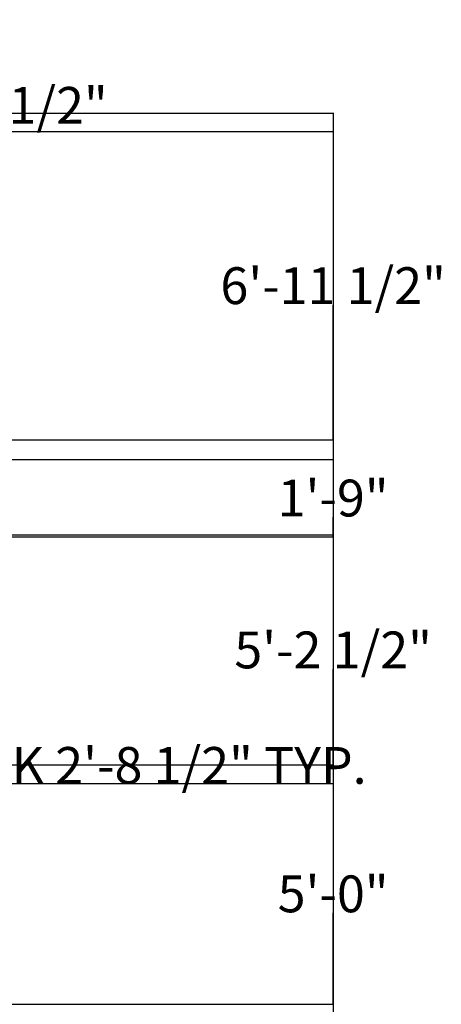
# Model space of a CAD drawing. Units: inches. Extents: x 541 to 1172, y -20 to 887.
# Tile 8 of 8: x 1058 to 1172, y 588 to 855. Entities that reach past the tile are written whole.
import ezdxf

# ---------------------------------------------------------------- set-up
doc = ezdxf.new("R2010")
doc.units = ezdxf.units.IN
doc.header["$MEASUREMENT"] = 0
doc.layers.add('A-ANNO-DIMS', color=2, linetype='Continuous', lineweight=18)
doc.styles.get("Standard").update_dxf_attribs({"font": 'arial.ttf'})
doc.dimstyles.get("Standard").update_dxf_attribs({"dimtxt": 10, "dimasz": 0.18, "dimexe": 0.18, "dimexo": 0.0625, "dimgap": 0.09, "dimtad": 0, "dimtih": 1, "dimtoh": 1, "dimdec": 1, "dimzin": 0, "dimdsep": 46, "dimlunit": 4, "dimtxsty": 'Standard', "dimcen": 0.09, "dimadec": 0, "dimazin": 0, "dimtfac": 1, "dimtdec": 1, "dimtofl": 0, "dimtmove": 0, "dimatfit": 3, "dimfxl": 1, "dimtolj": 1, "dimtzin": 0, "dimarcsym": 0})

# ---------------------------------------------------------------- blocks, each defined once
blk = doc.blocks.new('*D51')
at = {"layer": 'A-ANNO-DIMS', "color": 0, "lineweight": -2, "transparency": 16777216}
for p, q in [((999.81, 647.72), (999.81, 652.71)), ((999.99, 652.53), (1032.1, 652.53)), ((1032.28, 647.72), (1032.28, 652.71)), ((1032.28, 652.53), (1032.46, 652.53))]:
    blk.add_line(p, q, dxfattribs=at)
for points in [[(999.99, 652.56), (999.99, 652.5), (999.81, 652.53)], [(1032.1, 652.56), (1032.1, 652.5), (1032.28, 652.53)]]:
    blk.add_solid(points, dxfattribs=at)
at = {"layer": 'Defpoints', "color": 0, "lineweight": -2, "transparency": 16777216}
for p in [(1032.28, 652.53), (999.81, 647.65), (1032.28, 647.65)]:
    blk.add_point(p, dxfattribs=at)
at = {"layer": 'A-ANNO-DIMS', "color": 0, "transparency": 16777216, "insert": (1092.9, 652.53), "char_height": 10, "attachment_point": 5}
blk.add_mtext('\\A1;SINK 2\'-8 1/2" TYP.', dxfattribs=at)
blk = doc.blocks.new('*D53')
at = {"layer": 'A-ANNO-DIMS', "color": 0, "lineweight": -2, "transparency": 16777216}
for p, q in [((940.56, 824.91), (940.56, 831.98)), ((940.74, 831.8), (986.74, 831.8)), ((986.92, 824.91), (986.92, 831.98)), ((986.92, 831.8), (987.1, 831.8))]:
    blk.add_line(p, q, dxfattribs=at)
for points in [[(940.74, 831.83), (940.74, 831.77), (940.56, 831.8)], [(986.74, 831.83), (986.74, 831.77), (986.92, 831.8)]]:
    blk.add_solid(points, dxfattribs=at)
at = {"layer": 'Defpoints', "color": 0, "lineweight": -2, "transparency": 16777216}
for p in [(986.92, 831.8), (940.56, 824.85), (986.92, 824.85)]:
    blk.add_point(p, dxfattribs=at)
at = {"layer": 'A-ANNO-DIMS', "color": 0, "transparency": 16777216, "insert": (1034.24, 831.8), "char_height": 10, "attachment_point": 5}
blk.add_mtext('\\A1;SINK 3\'-10 1/2"', dxfattribs=at)
blk = doc.blocks.new('*D70')
at = {"layer": 'A-ANNO-DIMS', "color": 0, "lineweight": -2, "transparency": 16777216}
for p, q in [((1036.7, 829.68), (1143.21, 829.68)), ((1143.03, 829.5), (1143.03, 444.36)), ((1143.03, 48.83), (1143.03, 433.97)), ((1037.35, 48.65), (1143.21, 48.65))]:
    blk.add_line(p, q, dxfattribs=at)
for points in [[(1143, 829.5), (1143.06, 829.5), (1143.03, 829.68)], [(1143, 48.83), (1143.06, 48.83), (1143.03, 48.65)]]:
    blk.add_solid(points, dxfattribs=at)
at = {"layer": 'Defpoints', "color": 0, "lineweight": -2, "transparency": 16777216}
for p in [(1036.64, 829.68), (1037.28, 48.65), (1143.03, 48.65)]:
    blk.add_point(p, dxfattribs=at)
at = {"layer": 'A-ANNO-DIMS', "color": 0, "transparency": 16777216, "insert": (1143.03, 439.17), "char_height": 10, "attachment_point": 5}
blk.add_mtext('\\A1;65\'-1"', dxfattribs=at)
blk = doc.blocks.new('*D79')
at = {"layer": 'A-ANNO-DIMS', "color": 0, "lineweight": -2, "transparency": 16777216}
for p, q in [((1031.73, 824.68), (1143.21, 824.68)), ((1143.03, 824.5), (1143.03, 788.09)), ((1143.03, 741.17), (1143.03, 777.57)), ((1032.19, 740.99), (1143.21, 740.99))]:
    blk.add_line(p, q, dxfattribs=at)
for points in [[(1143, 824.5), (1143.06, 824.5), (1143.03, 824.68)], [(1143, 741.17), (1143.06, 741.17), (1143.03, 740.99)]]:
    blk.add_solid(points, dxfattribs=at)
at = {"layer": 'Defpoints', "color": 0, "lineweight": -2, "transparency": 16777216}
for p in [(1031.66, 824.68), (1032.13, 740.99), (1143.03, 740.99)]:
    blk.add_point(p, dxfattribs=at)
at = {"layer": 'A-ANNO-DIMS', "color": 0, "transparency": 16777216, "insert": (1143.03, 782.83), "char_height": 10, "attachment_point": 5}
blk.add_mtext('\\A1;6\'-11 1/2"', dxfattribs=at)
blk = doc.blocks.new('*D80')
at = {"layer": 'A-ANNO-DIMS', "color": 0, "lineweight": -2, "transparency": 16777216}
for p, q in [((1032.33, 715.15), (1143.21, 715.15)), ((1143.03, 714.97), (1143.03, 689.16)), ((1143.03, 652.83), (1143.03, 678.64)), ((1032.35, 652.65), (1143.21, 652.65))]:
    blk.add_line(p, q, dxfattribs=at)
for points in [[(1143, 714.97), (1143.06, 714.97), (1143.03, 715.15)], [(1143, 652.83), (1143.06, 652.83), (1143.03, 652.65)]]:
    blk.add_solid(points, dxfattribs=at)
at = {"layer": 'Defpoints', "color": 0, "lineweight": -2, "transparency": 16777216}
for p in [(1032.27, 715.15), (1032.28, 652.65), (1143.03, 652.65)]:
    blk.add_point(p, dxfattribs=at)
at = {"layer": 'A-ANNO-DIMS', "color": 0, "transparency": 16777216, "insert": (1143.03, 683.9), "char_height": 10, "attachment_point": 5}
blk.add_mtext('\\A1;5\'-2 1/2"', dxfattribs=at)
blk = doc.blocks.new('*D81')
at = {"layer": 'A-ANNO-DIMS', "color": 0, "lineweight": -2, "transparency": 16777216}
for p, q in [((1032.35, 647.65), (1143.21, 647.65)), ((1143.03, 647.47), (1143.03, 622.85)), ((1143.03, 587.83), (1143.03, 612.46)), ((1032.35, 587.65), (1143.21, 587.65))]:
    blk.add_line(p, q, dxfattribs=at)
for points in [[(1143, 647.47), (1143.06, 647.47), (1143.03, 647.65)], [(1143, 587.83), (1143.06, 587.83), (1143.03, 587.65)]]:
    blk.add_solid(points, dxfattribs=at)
at = {"layer": 'Defpoints', "color": 0, "lineweight": -2, "transparency": 16777216}
for p in [(1032.28, 647.65), (1032.28, 587.65), (1143.03, 587.65)]:
    blk.add_point(p, dxfattribs=at)
at = {"layer": 'A-ANNO-DIMS', "color": 0, "transparency": 16777216, "insert": (1143.03, 617.65), "char_height": 10, "attachment_point": 5}
blk.add_mtext('\\A1;5\'-0"', dxfattribs=at)
blk = doc.blocks.new('*D101')
at = {"layer": 'A-ANNO-DIMS', "color": 0, "lineweight": -2, "transparency": 16777216}
for p, q in [((805.35, 735.65), (1143.21, 735.65)), ((1143.03, 735.47), (1143.03, 730.35)), ((1143.03, 714.83), (1143.03, 719.96)), ((805.35, 714.65), (1143.21, 714.65))]:
    blk.add_line(p, q, dxfattribs=at)
for points in [[(1143, 735.47), (1143.06, 735.47), (1143.03, 735.65)], [(1143, 714.83), (1143.06, 714.83), (1143.03, 714.65)]]:
    blk.add_solid(points, dxfattribs=at)
at = {"layer": 'Defpoints', "color": 0, "lineweight": -2, "transparency": 16777216}
for p in [(805.28, 735.65), (1143.03, 735.65), (805.28, 714.65)]:
    blk.add_point(p, dxfattribs=at)
at = {"layer": 'A-ANNO-DIMS', "color": 0, "transparency": 16777216, "insert": (1143.03, 725.15), "char_height": 10, "attachment_point": 5}
blk.add_mtext('\\A1;1\'-9"', dxfattribs=at)

msp = doc.modelspace()

# ---------------------------------------------------------------- dimensions: what is measured, and where the dimension line sits
at = {"layer": 'A-ANNO-DIMS'}
for base, p1, p2, text, picture, middle in [((986.92, 831.8), (940.56, 824.85), (986.92, 824.85), 'SINK <>', '*D53', (1034.24, 831.8)), ((1032.28, 652.53), (999.81, 647.65), (1032.28, 647.65), 'SINK <> TYP.', '*D51', (1092.9, 652.53))]:
    dim = msp.add_linear_dim(base=base, p1=p1, p2=p2, text=text, dimstyle='Standard', override={"dimdec": 1, "dimlfac": 1, "dimrnd": 0, "dimzin": 1, "dimdsep": 46, "dimlunit": 4, "dimfrac": 2}, dxfattribs=at)
    dim.commit()
    dim.dimension.update_dxf_attribs({"geometry": picture, "text_midpoint": middle})
for base, p1, p2, picture, middle in [((1143.03, 48.65), (1036.64, 829.68), (1037.28, 48.65), '*D70', (1143.03, 439.17)), ((1143.03, 740.99), (1031.66, 824.68), (1032.13, 740.99), '*D79', (1143.03, 782.83)), ((1143.03, 735.65), (805.28, 714.65), (805.28, 735.65), '*D101', (1143.03, 725.15)), ((1143.03, 652.65), (1032.27, 715.15), (1032.28, 652.65), '*D80', (1143.03, 683.9)), ((1143.03, 587.65), (1032.28, 647.65), (1032.28, 587.65), '*D81', (1143.03, 617.65))]:
    dim = msp.add_linear_dim(base=base, p1=p1, p2=p2, angle=90, dimstyle='Standard', override={"dimdec": 1, "dimlfac": 1, "dimrnd": 0, "dimzin": 1, "dimdsep": 46, "dimlunit": 4, "dimfrac": 2}, dxfattribs=at)
    dim.commit()
    dim.dimension.update_dxf_attribs({"geometry": picture, "text_midpoint": middle})

doc.saveas('drawing.dxf')
